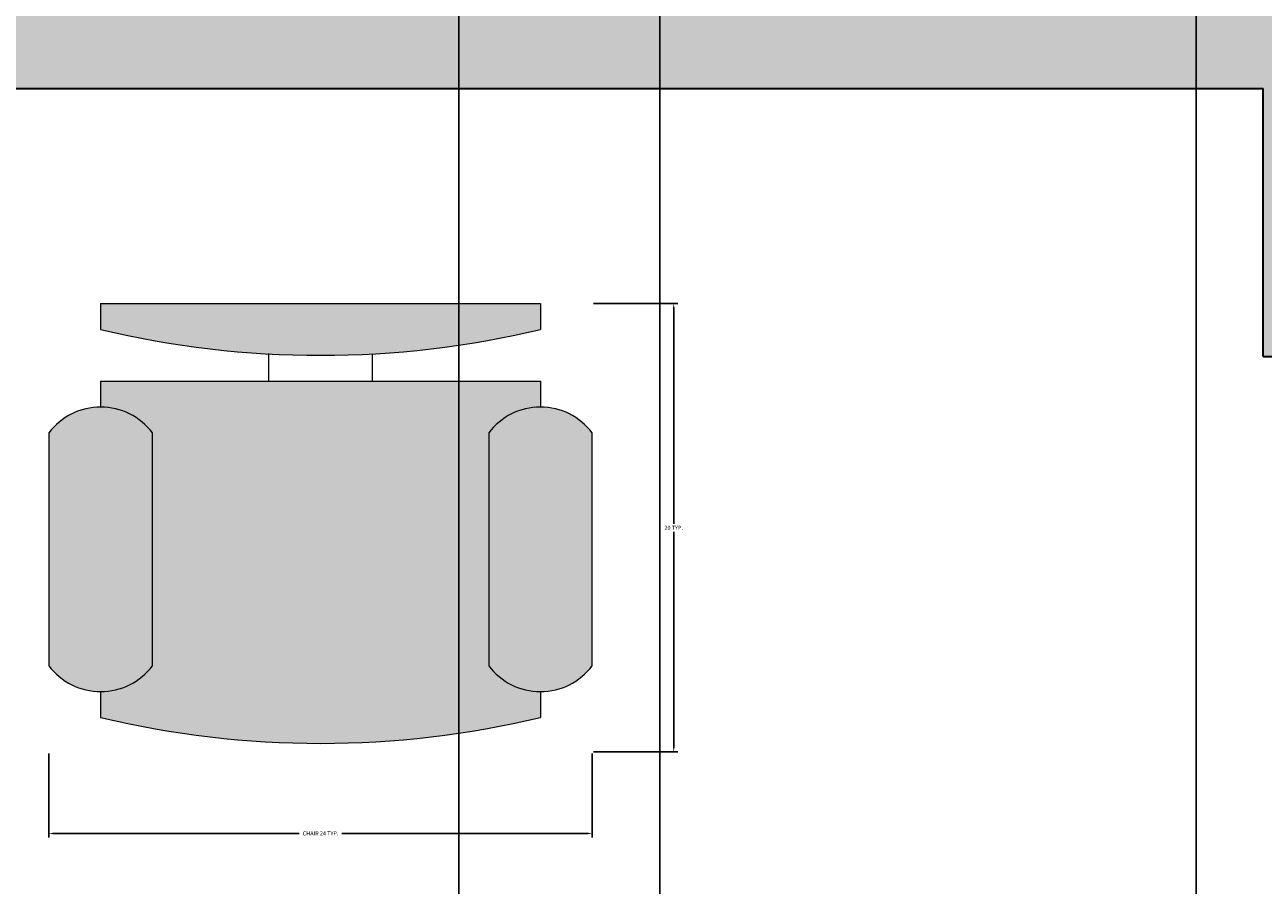
# Model space of a CAD drawing. Units: inches. Extents: x 1567 to 1964, y 1813 to 2447.
# Tile 12 of 28: x 1683 to 1738, y 2224 to 2262. Entities that reach past the tile are written whole.
import ezdxf

# ---------------------------------------------------------------- set-up
doc = ezdxf.new("R2010")
doc.units = ezdxf.units.IN
for name, color, linetype, lineweight in [('A-ANNO-DIMS', 2, 'Continuous', 18), ('A-FURN', 8, 'Continuous', 18), ('A-WALL', 7, 'Continuous', 35)]:
    doc.layers.add(name, color=color, linetype=linetype, lineweight=lineweight)
doc.layers.add('A-FURN-PATT', color=252, linetype='Continuous', lineweight=13, true_color=0x939598)
doc.layers.add('A-WALL-PATT', color=251, linetype='Continuous', lineweight=13, true_color=0x636466)
doc.styles.get("Standard").update_dxf_attribs({"font": 'arial.ttf'})
doc.dimstyles.get("Standard").update_dxf_attribs({"dimtxt": 0.18, "dimasz": 0.18, "dimexe": 0.18, "dimexo": 0.0625, "dimgap": 0.09, "dimtad": 0, "dimtih": 1, "dimtoh": 1, "dimdec": 4, "dimzin": 0, "dimdsep": 46, "dimtxsty": 'Standard', "dimcen": 0.09, "dimadec": 0, "dimazin": 0, "dimtfac": 1, "dimtdec": 4, "dimtofl": 0, "dimtmove": 0, "dimatfit": 3, "dimfxl": 1, "dimtolj": 1, "dimtzin": 0, "dimarcsym": 0})

# ---------------------------------------------------------------- blocks, each defined once
blk = doc.blocks.new('Chair - Desk')
for p, q in [((-8.5, 0), (-8.5, -1)), ((-8.5, 0), (8.5, 0)), ((8.5, 0), (8.5, -1)), ((-2, -3), (-2, -1.9355)), ((2, -1.9576), (2, -3)), ((-8.5, -3), (-8.5, -4)), ((-8.5, -3), (8.5, -3)), ((8.5, -3), (8.5, -4)), ((-10.5, -5), (-10.5, -14)), ((-6.5, -14), (-6.5, -5)), ((6.5, -5), (6.5, -14)), ((10.5, -14), (10.5, -5)), ((-8.5, -15), (-8.5, -16)), ((8.5, -15), (8.5, -16))]:
    blk.add_line(p, q)
for centre, radius, start, end in [((0, 34.625), 36.625, 256.5803, 283.4197), ((-8.5, -6.5), 2.5, 36.8699, 143.1301), ((8.5, -6.5), 2.5, 36.8699, 143.1301), ((-8.5, -12.5), 2.5, 216.8699, 323.1301), ((8.5, -12.5), 2.5, 216.8699, 323.1301), ((0, 19.625), 36.625, 256.5803, 283.4197)]:
    blk.add_arc(centre, radius, start, end)
blk = doc.blocks.new('*D21')
at = {"layer": 'A-ANNO-DIMS', "color": 0, "lineweight": -2, "transparency": 16777216}
for p, q in [((1684.094, 2229.533), (1684.094, 2225.769)), ((1708.404, 2229.533), (1708.404, 2225.769)), ((1684.274, 2225.949), (1695.296, 2225.949)), ((1708.224, 2225.949), (1697.202, 2225.949))]:
    blk.add_line(p, q, dxfattribs=at)
at = {"layer": 'A-ANNO-DIMS', "color": 0, "transparency": 16777216}
for points in [[(1684.274, 2225.979), (1684.274, 2225.919), (1684.094, 2225.949)], [(1708.224, 2225.979), (1708.224, 2225.919), (1708.404, 2225.949)]]:
    blk.add_solid(points, dxfattribs=at)
at = {"layer": 'Defpoints', "color": 0, "transparency": 16777216}
for p in [(1684.094, 2229.595), (1708.404, 2229.595), (1708.404, 2225.949)]:
    blk.add_point(p, dxfattribs=at)
at = {"layer": 'A-ANNO-DIMS', "color": 0, "transparency": 16777216, "insert": (1696.249, 2225.949), "char_height": 0.18, "attachment_point": 5}
blk.add_mtext('\\A1;CHAIR 24 TYP.', dxfattribs=at)
blk = doc.blocks.new('*D22')
at = {"layer": 'A-ANNO-DIMS', "color": 0, "lineweight": -2, "transparency": 16777216}
for p, q in [((1708.467, 2249.661), (1712.231, 2249.661)), ((1712.051, 2249.481), (1712.051, 2239.81)), ((1712.051, 2229.775), (1712.051, 2239.446)), ((1708.467, 2229.595), (1712.231, 2229.595))]:
    blk.add_line(p, q, dxfattribs=at)
at = {"layer": 'A-ANNO-DIMS', "color": 0, "transparency": 16777216}
for points in [[(1712.021, 2249.481), (1712.081, 2249.481), (1712.051, 2249.661)], [(1712.021, 2229.775), (1712.081, 2229.775), (1712.051, 2229.595)]]:
    blk.add_solid(points, dxfattribs=at)
at = {"layer": 'Defpoints', "color": 0, "transparency": 16777216}
for p in [(1708.404, 2249.661), (1712.051, 2249.661), (1708.404, 2229.595)]:
    blk.add_point(p, dxfattribs=at)
at = {"layer": 'A-ANNO-DIMS', "color": 0, "transparency": 16777216, "insert": (1712.051, 2239.628), "char_height": 0.18, "attachment_point": 5}
blk.add_mtext('\\A1;20 TYP.', dxfattribs=at)
blk = doc.blocks.new('*D54')
at = {"layer": 'A-ANNO-DIMS', "color": 0, "lineweight": -2, "transparency": 16777216}
for p, q in [((1711.43, 1964.352), (1711.43, 2447.12)), ((1711.61, 2446.94), (1753.211, 2446.94)), ((1795.25, 2446.94), (1753.648, 2446.94)), ((1795.43, 1964.352), (1795.43, 2447.12))]:
    blk.add_line(p, q, dxfattribs=at)
at = {"layer": 'A-ANNO-DIMS', "color": 0, "transparency": 16777216}
for points in [[(1711.61, 2446.97), (1711.61, 2446.91), (1711.43, 2446.94)], [(1795.25, 2446.97), (1795.25, 2446.91), (1795.43, 2446.94)]]:
    blk.add_solid(points, dxfattribs=at)
at = {"layer": 'Defpoints', "color": 0, "transparency": 16777216}
for p in [(1795.43, 2446.94), (1711.43, 1964.29), (1795.43, 1964.29)]:
    blk.add_point(p, dxfattribs=at)
at = {"layer": 'A-ANNO-DIMS', "color": 0, "transparency": 16777216, "insert": (1753.43, 2446.94), "char_height": 0.18, "attachment_point": 5}
blk.add_mtext('\\A1;84', dxfattribs=at)
blk = doc.blocks.new('*D60')
at = {"layer": 'A-ANNO-DIMS', "color": 0, "lineweight": -2, "transparency": 16777216}
for p, q in [((1660.43, 2063.352), (1660.43, 2447.12)), ((1660.61, 2446.94), (1681.208, 2446.94)), ((1702.25, 2446.94), (1681.651, 2446.94)), ((1702.43, 2063.352), (1702.43, 2447.12))]:
    blk.add_line(p, q, dxfattribs=at)
at = {"layer": 'A-ANNO-DIMS', "color": 0, "transparency": 16777216}
for points in [[(1660.61, 2446.97), (1660.61, 2446.91), (1660.43, 2446.94)], [(1702.25, 2446.97), (1702.25, 2446.91), (1702.43, 2446.94)]]:
    blk.add_solid(points, dxfattribs=at)
at = {"layer": 'Defpoints', "color": 0, "transparency": 16777216}
for p in [(1660.43, 2446.94), (1660.43, 2063.29), (1702.43, 2063.29)]:
    blk.add_point(p, dxfattribs=at)
at = {"layer": 'A-ANNO-DIMS', "color": 0, "transparency": 16777216, "insert": (1681.43, 2446.94), "char_height": 0.18, "attachment_point": 5}
blk.add_mtext('\\A1;42', dxfattribs=at)
blk = doc.blocks.new('*D63')
at = {"layer": 'A-ANNO-DIMS', "color": 0, "lineweight": -2, "transparency": 16777216}
for p, q in [((1735.43, 1988.352), (1735.43, 2447.12)), ((1735.61, 2446.94), (1753.211, 2446.94)), ((1771.25, 2446.94), (1753.648, 2446.94)), ((1771.43, 1988.352), (1771.43, 2447.12))]:
    blk.add_line(p, q, dxfattribs=at)
at = {"layer": 'A-ANNO-DIMS', "color": 0, "transparency": 16777216}
for points in [[(1735.61, 2446.97), (1735.61, 2446.91), (1735.43, 2446.94)], [(1771.25, 2446.97), (1771.25, 2446.91), (1771.43, 2446.94)]]:
    blk.add_solid(points, dxfattribs=at)
at = {"layer": 'Defpoints', "color": 0, "transparency": 16777216}
for p in [(1771.43, 2446.94), (1735.43, 1988.29), (1771.43, 1988.29)]:
    blk.add_point(p, dxfattribs=at)
at = {"layer": 'A-ANNO-DIMS', "color": 0, "transparency": 16777216, "insert": (1753.43, 2446.94), "char_height": 0.18, "attachment_point": 5}
blk.add_mtext('\\A1;36', dxfattribs=at)
blk = doc.blocks.new('*D64')
at = {"layer": 'A-ANNO-DIMS', "color": 0, "lineweight": -2, "transparency": 16777216}
for p, q in [((1711.43, 2055.852), (1711.43, 2447.12)), ((1711.61, 2446.94), (1723.209, 2446.94)), ((1735.25, 2446.94), (1723.65, 2446.94)), ((1735.43, 2055.852), (1735.43, 2447.12))]:
    blk.add_line(p, q, dxfattribs=at)
at = {"layer": 'A-ANNO-DIMS', "color": 0, "transparency": 16777216}
for points in [[(1711.61, 2446.97), (1711.61, 2446.91), (1711.43, 2446.94)], [(1735.25, 2446.97), (1735.25, 2446.91), (1735.43, 2446.94)]]:
    blk.add_solid(points, dxfattribs=at)
at = {"layer": 'Defpoints', "color": 0, "transparency": 16777216}
for p in [(1735.43, 2446.94), (1711.43, 2055.79), (1735.43, 2055.79)]:
    blk.add_point(p, dxfattribs=at)
at = {"layer": 'A-ANNO-DIMS', "color": 0, "transparency": 16777216, "insert": (1723.43, 2446.94), "char_height": 0.18, "attachment_point": 5}
blk.add_mtext('\\A1;24', dxfattribs=at)

msp = doc.modelspace()

# ---------------------------------------------------------------- hatches: boundary and pattern name
at = {"layer": 'A-FURN-PATT'}
h = msp.add_hatch(color=256, dxfattribs=at)
h.dxf.hatch_style = 1
h.paths.add_polyline_path([(1621.2532, 2242.0229), (1643.7811, 2241.7239), (1643.8607, 2247.7234), (1617.863, 2248.0685, 0.1904762), (1616.7481, 2164.0759), (1642.7458, 2163.7308), (1642.8254, 2169.7302), (1620.2975, 2170.0293, -0.1519478)])
h.paths.add_polyline_path([(1673.5306, 2249.6607), (1653.8509, 2249.6607), (1653.8509, 2248.5031, 0.1176471), (1673.5306, 2248.5031)])
h.paths.add_polyline_path([(1706.0889, 2249.6607), (1686.4092, 2249.6607), (1686.4092, 2248.5031, 0.1176471), (1706.0889, 2248.5031)])
h.paths.add_polyline_path([(1782.4511, 2227.4197), (1766.4511, 2227.4197), (1766.2949, 2226.4197), (1782.6074, 2226.4197)])
h.paths.add_polyline_path([(1810.4511, 2227.4197), (1794.4511, 2227.4197), (1794.2949, 2226.4197), (1810.6074, 2226.4197)])
h.paths.add_polyline_path([(1743.9511, 2208.076), (1742.9511, 2207.9197), (1742.9511, 2191.9197), (1743.9511, 2191.7635)])
h.paths.add_polyline_path([(1782.6074, 2173.4197), (1766.2949, 2173.4197), (1766.4511, 2172.4197), (1782.4511, 2172.4197)])
h.paths.add_polyline_path([(1810.6074, 2173.4197), (1794.2949, 2173.4197), (1794.4511, 2172.4197), (1810.4511, 2172.4197)])
h.paths.add_polyline_path([(1861.053, 2006.5071), (1845.8531, 2006.5071), (1861.053, 1991.3071)])
h.paths.add_polyline_path([(1905.853, 1993.7071), (1861.053, 1993.7071), (1861.053, 1991.3071), (1905.853, 1991.3071)])
h.paths.add_polyline_path([(1919.7245, 2257.29, 0.5000001), (1918.7245, 2258.29), (1901.7245, 2258.29, 0.5000001), (1900.7245, 2257.29), (1900.7245, 2253.29, 0.5000001), (1901.7245, 2252.29), (1918.7245, 2252.29, 0.5000001), (1919.7245, 2253.29)])
h.paths.add_polyline_path([(1875.9094, 2391.0204), (1875.9094, 2375.8204), (1891.1093, 2375.8204)], flags=17)
h.paths.add_polyline_path([(1891.1093, 2405.4204), (1831.1094, 2405.4204), (1831.1094, 2391.0204), (1839.1093, 2391.0204), (1839.1093, 2404.2204), (1859.9093, 2404.2204), (1859.9093, 2391.0204), (1862.3093, 2391.0204), (1862.3093, 2404.2204), (1883.1093, 2404.2204), (1883.1093, 2389.0204), (1877.9094, 2389.0204), (1891.1093, 2375.8204)])
h.paths.add_polyline_path([(1682.1402, 2390.0316), (1682.1402, 2374.8316), (1697.3402, 2374.8316)], flags=17)
h.paths.add_polyline_path([(1697.3402, 2404.4316), (1637.3402, 2404.4316), (1637.3402, 2390.0316), (1645.3402, 2390.0316), (1645.3402, 2403.2316), (1666.1402, 2403.2316), (1666.1402, 2390.0316), (1668.5402, 2390.0316), (1668.5402, 2403.2316), (1689.3402, 2403.2316), (1689.3402, 2388.0316), (1684.1402, 2388.0316), (1697.3402, 2374.8316)])
h = msp.add_hatch(color=256, dxfattribs=at)
h.dxf.hatch_style = 1
h.paths.add_polyline_path([(1642.2233, 2241.7446), (1623.1648, 2241.9976), (1622.8462, 2217.9997), (1641.9047, 2217.7467)])
h.paths.add_polyline_path([(1641.9047, 2217.7467), (1622.8462, 2217.9997), (1622.5277, 2194.0018), (1641.5862, 2193.7488)])
h.paths.add_polyline_path([(1641.5862, 2193.7488), (1622.5277, 2194.0018), (1622.2091, 2170.0039), (1641.2677, 2169.7509)])
h.paths.add_polyline_path([(1671.2154, 2243.8726, -0.236068), (1673.5306, 2245.0302), (1673.5306, 2246.1879), (1653.8509, 2246.1879), (1653.8509, 2245.0302, -0.236068), (1656.1662, 2243.8726), (1656.1662, 2233.4539, -0.236068), (1653.8509, 2232.2963), (1653.8509, 2231.1387, 0.1176471), (1673.5306, 2231.1387), (1673.5306, 2232.2963, -0.236068), (1671.2154, 2233.4539)])
h.paths.add_polyline_path([(1703.7736, 2243.8726, -0.236068), (1706.0889, 2245.0302), (1706.0889, 2246.1879), (1686.4092, 2246.1879), (1686.4092, 2245.0302, -0.236068), (1688.7245, 2243.8726), (1688.7245, 2233.4539, -0.236068), (1686.4092, 2232.2963), (1686.4092, 2231.1387, 0.1176471), (1706.0889, 2231.1387), (1706.0889, 2232.2963, -0.236068), (1703.7736, 2233.4539)])
h.paths.add_polyline_path([(1782.6855, 2225.9197), (1766.2168, 2225.9197), (1764.9668, 2217.9197), (1783.9356, 2217.9197)])
h.paths.add_polyline_path([(1810.6855, 2225.9197), (1794.2168, 2225.9197), (1792.9668, 2217.9197), (1811.9356, 2217.9197)])
h.paths.add_polyline_path([(1752.4511, 2209.4041), (1744.4511, 2208.1541), (1744.4511, 2191.6853), (1752.4511, 2190.4354)])
h.paths.add_polyline_path([(1783.9356, 2181.9197), (1764.9668, 2181.9197), (1766.2168, 2173.9197), (1782.6855, 2173.9197)])
h.paths.add_polyline_path([(1811.9356, 2181.9197), (1792.9668, 2181.9197), (1794.2168, 2173.9197), (1810.6855, 2173.9197)])
h.paths.add_polyline_path([(1832.4511, 2208.1541), (1824.4511, 2209.4041), (1824.4511, 2190.4354), (1832.4511, 2191.6853)])
h.paths.add_polyline_path([(1824.4511, 2194.4197), (1823.8775, 2194.266), (1823.2838, 2194.1743), (1822.6735, 2194.1363), (1822.0501, 2194.1437), (1821.4169, 2194.1882), (1820.7773, 2194.2615), (1820.1348, 2194.3554), (1819.4928, 2194.4614), (1818.8527, 2194.5726), (1818.2083, 2194.6873), (1817.5511, 2194.8049), (1816.873, 2194.9249), (1816.1656, 2195.0469), (1815.4205, 2195.1704), (1814.6296, 2195.2948), (1813.7845, 2195.4197), (1812.88, 2195.5442), (1811.9238, 2195.6658), (1810.9265, 2195.7815), (1809.899, 2195.8885), (1808.852, 2195.9837), (1807.7962, 2196.0643), (1806.7423, 2196.1273), (1805.7011, 2196.1697), (1804.6806, 2196.1896), (1803.6777, 2196.188), (1802.6865, 2196.1668), (1801.7011, 2196.1281), (1800.7158, 2196.0737), (1799.7245, 2196.0057), (1798.7216, 2195.9259), (1797.7011, 2195.8364), (1796.6564, 2195.7387), (1795.5781, 2195.6333), (1794.4557, 2195.52), (1793.2792, 2195.3989), (1792.0383, 2195.27), (1790.7226, 2195.1333), (1789.3219, 2194.9887), (1787.8261, 2194.8364), (1786.1882, 2194.6764), (1784.2148, 2194.5096), (1781.6759, 2194.3369), (1778.3417, 2194.1593), (1773.9821, 2193.9778), (1768.3671, 2193.7934), (1761.2668, 2193.6071), (1752.4511, 2193.4197), (1752.4511, 2189.9197), (1762.0489, 2190.1067), (1769.9836, 2190.2908), (1776.4672, 2190.469), (1781.7115, 2190.6385), (1785.9285, 2190.7962), (1789.33, 2190.9393), (1792.128, 2191.0648), (1794.5344, 2191.1697), (1796.7278, 2191.2521), (1798.7532, 2191.313), (1800.6223, 2191.3543), (1802.3469, 2191.3781), (1803.9387, 2191.3862), (1805.4094, 2191.3807), (1806.7708, 2191.3634), (1808.0345, 2191.3364), (1809.2127, 2191.3013), (1810.3196, 2191.2589), (1811.3699, 2191.2097), (1812.3782, 2191.1541), (1813.3592, 2191.0927), (1814.3274, 2191.0259), (1815.2976, 2190.9542), (1816.2845, 2190.8781), (1817.2985, 2190.7986), (1818.3339, 2190.7186), (1819.3811, 2190.6415), (1820.4303, 2190.5708), (1821.4716, 2190.5098), (1822.4954, 2190.4621), (1823.4918, 2190.4309), (1824.3581, 2190.4208), (1824.4511, 2190.4354)])
h.paths.add_polyline_path([(1874.6531, 1991.3071), (1861.053, 1991.3071), (1859.053, 1993.3071), (1853.8531, 1993.3071), (1853.8531, 1978.1071), (1874.6531, 1978.1071)], flags=17)
h.paths.add_polyline_path([(1897.8531, 1991.3071), (1877.0531, 1991.3071), (1877.0531, 1978.1071), (1897.8531, 1978.1071)], flags=17)
h.paths.add_polyline_path([(1853.8531, 1993.3071), (1859.053, 1993.3071), (1845.8531, 2006.5071), (1845.8531, 1976.9071), (1905.853, 1976.9071), (1905.853, 1991.3071), (1897.8531, 1991.3071), (1897.8531, 1978.1071), (1877.0531, 1978.1071), (1877.0531, 1991.3071), (1874.6531, 1991.3071), (1874.6531, 1978.1071), (1853.8531, 1978.1071)])
h.paths.add_polyline_path([(1920.7245, 2259.29), (1899.7245, 2259.29), (1899.7245, 2251.29), (1920.7245, 2251.29)])
h.paths.add_polyline_path([(1918.7245, 2252.29, 0.5000001), (1919.7245, 2253.29), (1919.7245, 2257.29, 0.5000001), (1918.7245, 2258.29), (1901.7245, 2258.29, 0.5000001), (1900.7245, 2257.29), (1900.7245, 2253.29, 0.5000001), (1901.7245, 2252.29)], flags=16)
h.paths.add_polyline_path([(1843.2327, 2065.967), (1919.26, 2065.967), (1919.26, 2095.8187), (1843.2327, 2095.8187)], flags=9)
h = msp.add_hatch(color=256, dxfattribs=at)
h.dxf.hatch_style = 1
h.paths.add_polyline_path([(1622.8462, 2217.9997), (1616.0605, 2218.0897, 0.0496282), (1615.7419, 2194.0919), (1622.5277, 2194.0018)])
h.paths.add_polyline_path([(1623.1648, 2241.9976), (1621.2532, 2242.0229, 0.0506467), (1616.0605, 2218.0897), (1622.8462, 2217.9997)])
h.paths.add_polyline_path([(1622.5277, 2194.0018), (1615.7419, 2194.0919, 0.0506466), (1620.2975, 2170.0293), (1622.2091, 2170.0039)])
h.paths.add_polyline_path([(1656.1662, 2243.8726, 0.5), (1651.5357, 2243.8726), (1651.5357, 2233.4539, 0.5), (1656.1662, 2233.4539)])
h.paths.add_polyline_path([(1675.8459, 2243.8726, 0.5), (1671.2154, 2243.8726), (1671.2154, 2233.4539, 0.5), (1675.8459, 2233.4539)])
h.paths.add_polyline_path([(1688.7245, 2243.8726, 0.5), (1684.094, 2243.8726), (1684.094, 2233.4539, 0.5), (1688.7245, 2233.4539)])
h.paths.add_polyline_path([(1708.4042, 2243.8726, 0.5), (1703.7736, 2243.8726), (1703.7736, 2233.4539, 0.5), (1708.4042, 2233.4539)])
at = {"layer": 'A-WALL-PATT'}
h = msp.add_hatch(color=256, dxfattribs=at)
h.dxf.hatch_style = 1
h.paths.add_polyline_path([(1606.4295, 2407.29), (1654.4295, 2407.29), (1654.4295, 2416.29), (1597.4295, 2416.29), (1597.4295, 2217.29), (1606.4295, 2217.29), (1606.4295, 2259.29), (1738.4295, 2259.29), (1738.4295, 2247.29), (1742.4295, 2247.29), (1742.4295, 2259.29), (1742.4295, 2272.29), (1738.4295, 2272.29), (1738.4295, 2263.29), (1606.4295, 2263.29)])
h.paths.add_polyline_path([(1753.4295, 2416.29), (1690.4295, 2416.29), (1690.4295, 2407.29), (1738.4295, 2407.29), (1738.4295, 2308.29), (1742.4295, 2308.29), (1742.4295, 2331.29), (1746.9295, 2331.29), (1746.9295, 2335.29), (1742.4295, 2335.29), (1742.4295, 2407.29), (1753.4295, 2407.29)])
h.paths.add_polyline_path([(1840.4295, 2416.29), (1777.4295, 2416.29), (1777.4295, 2407.29), (1788.4295, 2407.29), (1788.4295, 2335.29), (1776.9295, 2335.29), (1776.9295, 2331.29), (1788.4295, 2331.29), (1788.4295, 2308.29), (1792.4295, 2308.29), (1792.4295, 2407.29), (1840.4295, 2407.29)])
h.paths.add_polyline_path([(1933.4295, 2416.29), (1876.4295, 2416.29), (1876.4295, 2407.29), (1924.4295, 2407.29), (1924.4295, 2263.29), (1792.4295, 2263.29), (1792.4295, 2272.29), (1788.4295, 2272.29), (1788.4295, 2259.29), (1872.4295, 2259.29), (1872.4295, 2171.29), (1880.9295, 2171.29), (1880.9295, 2175.29), (1876.4295, 2175.29), (1876.4295, 2259.29), (1924.4295, 2259.29), (1924.4295, 2229.29), (1933.4295, 2229.29)])
h.paths.add_polyline_path([(1933.4295, 2205.29), (1924.4295, 2205.29), (1924.4295, 2175.29), (1910.9295, 2175.29), (1910.9295, 2171.29), (1924.4295, 2171.29), (1924.4295, 2127.29), (1844.4295, 2127.29), (1844.4295, 2123.29), (1924.4295, 2123.29), (1924.4295, 2063.29), (1933.4295, 2063.29)])
h.paths.add_polyline_path([(1799.4295, 2123.29), (1808.4295, 2123.29), (1808.4295, 2127.29), (1781.4295, 2127.29), (1781.4295, 2123.29), (1795.4295, 2123.29), (1795.4295, 1964.29), (1711.4295, 1964.29), (1711.4295, 2123.29), (1751.4295, 2123.29), (1751.4295, 2127.29), (1742.4295, 2127.29), (1742.4295, 2139.29), (1738.4295, 2139.29), (1738.4295, 2127.29), (1678.4295, 2127.29), (1678.4295, 2123.29), (1702.4295, 2123.29), (1702.4295, 1913.29), (1678.4295, 1913.29), (1678.4295, 1904.29), (1711.4295, 1904.29), (1711.4295, 1960.29), (1795.4295, 1960.29), (1795.4295, 1906.69), (1929.4295, 1906.69), (1929.4295, 1848.29), (1601.4295, 1848.29), (1601.4295, 1904.29), (1630.4295, 1904.29), (1630.4295, 1913.29), (1606.4295, 1913.29), (1606.4295, 2123.29), (1630.4295, 2123.29), (1630.4295, 2127.29), (1606.4295, 2127.29), (1606.4295, 2169.29), (1597.4295, 2169.29), (1597.4295, 1844.29), (1933.4295, 1844.29), (1933.4295, 2027.29), (1924.4295, 2027.29), (1924.4295, 1967.29), (1833.9295, 1967.29), (1833.9295, 1963.29), (1924.4295, 1963.29), (1924.4295, 1910.69), (1799.4295, 1910.69), (1799.4295, 1963.29), (1803.9295, 1963.29), (1803.9295, 1967.29), (1799.4295, 1967.29)])

# ---------------------------------------------------------------- linework, layer by layer
at = {"layer": 'A-WALL'}
for p, q in [((1606.4295, 2259.29), (1738.4295, 2259.29)), ((1738.4295, 2247.29), (1738.4295, 2259.29)), ((1738.4295, 2247.29), (1742.4295, 2247.29))]:
    msp.add_line(p, q, dxfattribs=at)

# ---------------------------------------------------------------- block references
at = {"layer": 'A-FURN', "xscale": 1.157629009682769, "yscale": 1.157629009682769, "zscale": 1.157629009682769}
msp.add_blockref('Chair - Desk', (1696.2491, 2249.6607), dxfattribs=at)

# ---------------------------------------------------------------- dimensions: what is measured, and where the dimension line sits
at = {"layer": 'A-ANNO-DIMS'}
for base, p1, p2, picture, middle in [((1660.4295, 2446.94), (1702.4295, 2063.29), (1660.4295, 2063.29), '*D60', (1681.4295, 2446.94)), ((1795.4295, 2446.94), (1711.4295, 1964.29), (1795.4295, 1964.29), '*D54', (1753.4295, 2446.94)), ((1735.4295, 2446.94), (1711.4295, 2055.79), (1735.4295, 2055.79), '*D64', (1723.4295, 2446.94)), ((1771.4295, 2446.94), (1735.4295, 1988.29), (1771.4295, 1988.29), '*D63', (1753.4295, 2446.94))]:
    dim = msp.add_linear_dim(base=base, p1=p1, p2=p2, dimstyle='Standard', override={"dimdec": 0, "dimlfac": 1, "dimrnd": 0, "dimzin": 0, "dimdsep": 46, "dimlunit": 2}, dxfattribs=at)
    dim.commit()
    dim.dimension.update_dxf_attribs({"geometry": picture, "text_midpoint": middle})
dim = msp.add_linear_dim(base=(1712.0507, 2249.6607), p1=(1708.4042, 2229.5952), p2=(1708.4042, 2249.6607), angle=90, text='<> TYP.', dimstyle='Standard', override={"dimdec": 0, "dimlfac": 1, "dimrnd": 0, "dimzin": 0, "dimdsep": 46, "dimlunit": 2}, dxfattribs=at)
dim.commit()
dim.dimension.update_dxf_attribs({"geometry": '*D22', "text_midpoint": (1712.0507, 2239.628)})
dim = msp.add_linear_dim(base=(1708.4042, 2225.9486), p1=(1684.094, 2229.5952), p2=(1708.4042, 2229.5952), text='CHAIR <> TYP.', dimstyle='Standard', override={"dimdec": 0, "dimlfac": 1, "dimrnd": 0, "dimzin": 0, "dimdsep": 46, "dimlunit": 2}, dxfattribs=at)
dim.commit()
dim.dimension.update_dxf_attribs({"geometry": '*D21', "text_midpoint": (1696.2491, 2225.9486)})

doc.saveas('drawing.dxf')
